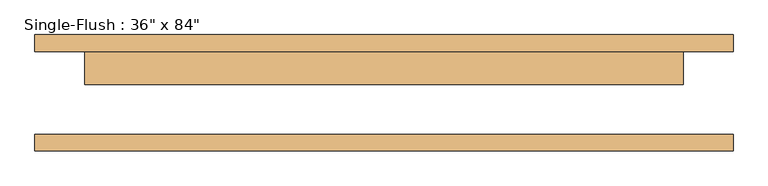
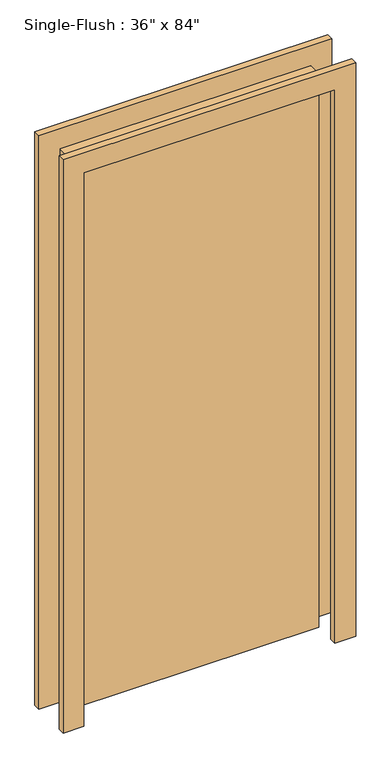
"""IFC4 building model written with IfcOpenShell, lengths in millimetres: door geometry."""

from ifc_helpers import new_model, si_unit, frame, origin, origin_with_axes, place, context, project, spatial, polyline, outline, extrude, source, transform, mapped, element, save


def door_a1797ceb(model_context):
    return source(origin(), model_context, "Body", "SweptSolid", [
        extrude(outline(polyline([(2209.8, -533.4), (0.0, -533.4), (0.0, -457.2), (2133.6, -457.2), (2133.6, 457.2), (0.0, 457.2), (0.0, 533.4), (2209.8, 533.4), (2209.8, -533.4)])), frame((0.0, 63.5, 0.0), z_axis=(0.0, 1.0, 0.0), x_axis=(0.0, 0.0, 1.0)), (0.0, 0.0, 1.0), 25.4),
        extrude(outline(polyline([(2209.8, 533.4), (2209.8, -533.4), (0.0, -533.4), (0.0, -457.2), (2133.6, -457.2), (2133.6, 457.2), (0.0, 457.2), (0.0, 533.4), (2209.8, 533.4)])), frame((0.0, -88.9, 0.0), z_axis=(0.0, 1.0, 0.0), x_axis=(0.0, 0.0, 1.0)), (0.0, 0.0, 1.0), 25.4),
        extrude(outline(polyline([(457.2, 12.7), (-457.2, 12.7), (-457.2, 63.5), (457.2, 63.5), (457.2, 12.7)])), origin_with_axes(), (0.0, 0.0, 1.0), 2133.6),
    ])


if __name__ == "__main__":
    model = new_model("IFC4")
    model_context = context("Model", 3, world=origin())
    ifc_project = project(units=[si_unit("LENGTHUNIT", "METRE", prefix="MILLI")], contexts=[model_context])
    site = spatial("IfcSite", under=ifc_project)
    building = spatial("IfcBuilding", under=site)
    placement = place(None, origin())
    door_shape = door_a1797ceb(model_context)
    element("IfcDoor", 1, ObjectType="Single-Flush : 36\" x 84\"", at=placement, inside=building, context=model_context, shape_type="MappedRepresentation", body=[
        mapped(door_shape, transform((0.0, 0.0, 0.0), x_axis=(1.0, 0.0, 0.0), y_axis=(0.0, 1.0, 0.0), z_axis=(0.0, 0.0, 1.0))),
    ])
    save(model, "model.ifc")

# Revit data of these elements
# Type "Single-Flush : 36\" x 84\""
#   Type Mark = "1"
#   Construction Type Id = "MDOOR"
#   Assembly Code = "C1020"
#   Analytic Construction = "Metal"
#   Thickness = 0' - 2"
#   Heat Transfer Coefficient (U) = 0.651978 BTU/(h·ft²·°F)
#   Height = 7' - 0"
#   Trim Projection Ext = 0' - 1"
#   Trim Projection Int = 0' - 1"
#   Trim Width = 0' - 3"
#   Width = 3' - 0"
#   Define Thermal Properties by = 1
#   Define Thermal Properties by = 1
#   Door Material = Door - Panel
#   Frame Material = Door - Frame
#   Visual Light Transmittance = 0
#   Solar Heat Gain Coefficient = 0
#   Function = (empty or 0)
#   Wall Closure = (empty or 0)
# Element 1 (IfcDoor, "Single-Flush : 36\" x 84\"")
#   Materials on its faces: "Door - Frame", "Door - Panel"
# Materials
#   "Door - Panel": class "Wood", colour RGB 210 159 95, transparency 0, Cost = 0
#   "Door - Frame": colour RGB 118 70 51, transparency 0, Cost = 0
